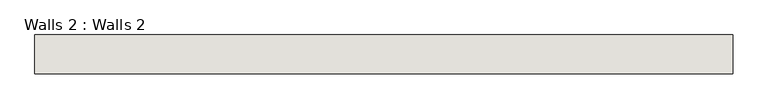
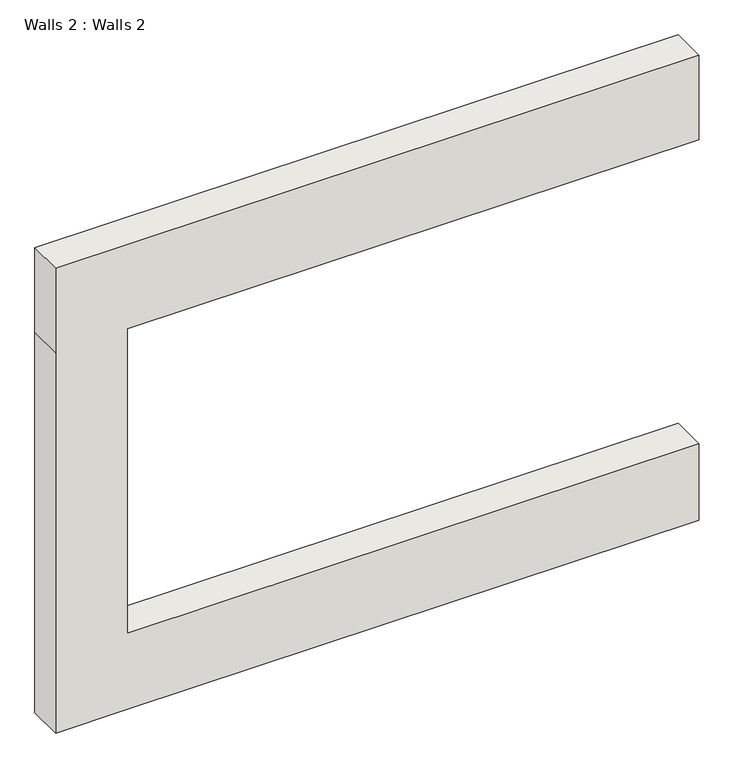
"""IFC4 building model written with IfcOpenShell, lengths in millimetres: wall geometry, Walls 2 : Walls 2."""

from ifc_helpers import new_model, si_unit, frame, origin, place, context, project, spatial, polyline, outline, extrude, source, transform, mapped, element, save


def walls_2_walls_2_451c460c(model_context):
    return source(origin(), model_context, "Body", "SweptSolid", [
        extrude(outline(polyline([(10746.7875846, -8246.7304753), (10746.7875846, -3369.9304753), (11505.4183492, -3369.9304753), (11505.4183492, -8856.3304753), (10746.7875846, -8856.3304753), (7315.2, -8856.3304753), (7315.2, -8246.7304753), (7315.2, -3369.9304753), (8001.5630935, -3369.9304753), (8001.5630935, -8246.7304753), (10746.7875846, -8246.7304753)])), frame((0.0, 2754.0297737, 0.0), z_axis=(0.0, 1.0, 0.0), x_axis=(0.0, 0.0, 1.0)), (0.0, 0.0, 1.0), 304.8),
    ])


if __name__ == "__main__":
    model = new_model("IFC4")
    model_context = context("Model", 3, world=origin())
    ifc_project = project(units=[si_unit("LENGTHUNIT", "METRE", prefix="MILLI")], contexts=[model_context])
    site = spatial("IfcSite", under=ifc_project)
    building = spatial("IfcBuilding", under=site)
    placement = place(None, origin())
    walls_2_walls_2_shape = walls_2_walls_2_451c460c(model_context)
    element("IfcWall", 1, ObjectType="Walls 2 : Walls 2", at=placement, inside=building, context=model_context, shape_type="MappedRepresentation", body=[
        mapped(walls_2_walls_2_shape, transform((0.0, 0.0, 0.0), x_axis=(1.0, 0.0, 0.0), y_axis=(0.0, 1.0, 0.0), z_axis=(0.0, 0.0, 1.0))),
    ])
    save(model, "model.ifc")

# Revit data of these elements
# Element 1 (IfcWall, "Walls 2 : Walls 2")
#   Materials on its faces: "Default Wall"
# Materials
#   "Default Wall": colour RGB 128 128 128, transparency 0
